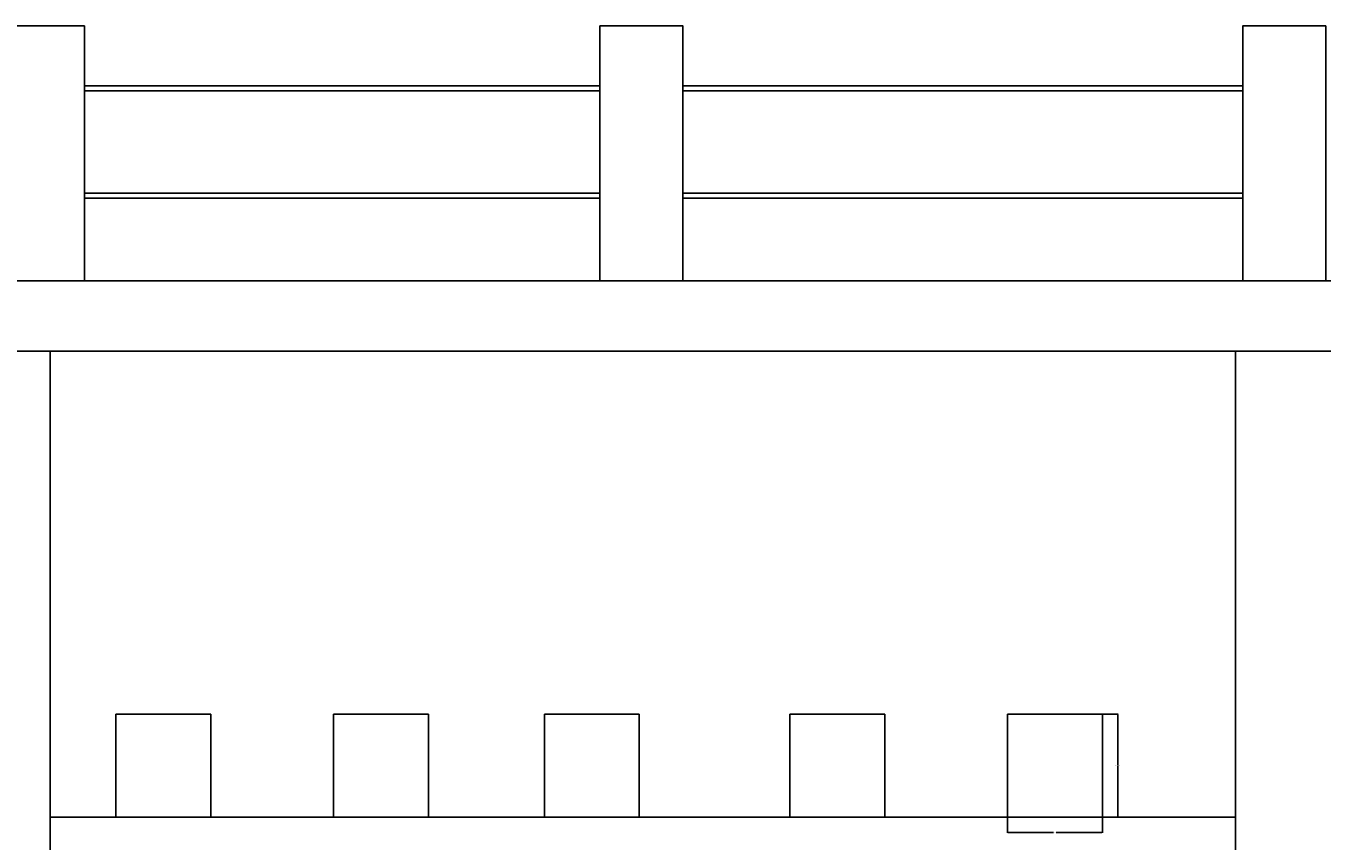
# Model space of a CAD drawing. Units: metres. Extents: x 10365 to 12529, y 3661 to 6248.
# Tile 8 of 9: x 11333 to 11858, y 5918 to 6248. Entities that reach past the tile are written whole.
import ezdxf

# ---------------------------------------------------------------- set-up
doc = ezdxf.new("R2010")
doc.units = ezdxf.units.M
doc.header["$MEASUREMENT"] = 0
doc.layers.add('A-ANNO-DIMS', color=2, linetype='Continuous', lineweight=18)
doc.layers.add('A-ELEV', color=7, linetype='Continuous', lineweight=25)
doc.styles.get("Standard").update_dxf_attribs({"font": 'arial.ttf'})
doc.dimstyles.get("Standard").update_dxf_attribs({"dimtxt": 0.18, "dimasz": 0.18, "dimexe": 0.18, "dimexo": 0.0625, "dimgap": 0.09, "dimtad": 0, "dimtih": 1, "dimtoh": 1, "dimdec": 0, "dimzin": 0, "dimdsep": 46, "dimtxsty": 'Standard', "dimcen": 0.09, "dimadec": 0, "dimazin": 0, "dimtfac": 1, "dimtdec": 0, "dimtofl": 0, "dimtmove": 0, "dimatfit": 3, "dimfxl": 1, "dimtolj": 1, "dimtzin": 0, "dimarcsym": 0})

# ---------------------------------------------------------------- blocks, each defined once
blk = doc.blocks.new('ELEV-PARAPET-BLOCK')
for p, q in [((0, 0), (0, 41.76)), ((0, 41.76), (38.46, 41.76)), ((38.46, 41.76), (38.46, 0))]:
    blk.add_line(p, q)
blk = doc.blocks.new('*D31')
at = {"layer": 'A-ANNO-DIMS', "color": 0, "lineweight": -2, "transparency": 16777216}
for p, q in [((11769.44, 5969.19), (11775.82, 5969.19)), ((11775.64, 5969.01), (11775.64, 5948.49)), ((11775.64, 5927.61), (11775.64, 5948.12)), ((11769.44, 5927.43), (11775.82, 5927.43))]:
    blk.add_line(p, q, dxfattribs=at)
at = {"layer": 'A-ANNO-DIMS', "color": 0, "transparency": 16777216}
for points in [[(11775.61, 5969.01), (11775.67, 5969.01), (11775.64, 5969.19)], [(11775.61, 5927.61), (11775.67, 5927.61), (11775.64, 5927.43)]]:
    blk.add_solid(points, dxfattribs=at)
at = {"layer": 'Defpoints', "color": 0, "transparency": 16777216}
for p in [(11769.38, 5969.19), (11775.64, 5969.19), (11769.38, 5927.43)]:
    blk.add_point(p, dxfattribs=at)
at = {"layer": 'A-ANNO-DIMS', "color": 0, "transparency": 16777216, "insert": (11775.64, 5948.31), "char_height": 0.18, "attachment_point": 5}
blk.add_mtext('\\A1;PARAPET BLOCK 42 TYP.', dxfattribs=at)
blk = doc.blocks.new('*D32')
at = {"layer": 'A-ANNO-DIMS', "color": 0, "lineweight": -2, "transparency": 16777216}
for p, q in [((11730.92, 5927.36), (11730.92, 5920.98)), ((11769.38, 5927.36), (11769.38, 5920.98)), ((11731.1, 5921.16), (11749.62, 5921.16)), ((11769.2, 5921.16), (11750.68, 5921.16))]:
    blk.add_line(p, q, dxfattribs=at)
at = {"layer": 'A-ANNO-DIMS', "color": 0, "transparency": 16777216}
for points in [[(11731.1, 5921.19), (11731.1, 5921.13), (11730.92, 5921.16)], [(11769.2, 5921.19), (11769.2, 5921.13), (11769.38, 5921.16)]]:
    blk.add_solid(points, dxfattribs=at)
at = {"layer": 'Defpoints', "color": 0, "transparency": 16777216}
for p in [(11730.92, 5927.43), (11769.38, 5927.43), (11769.38, 5921.16)]:
    blk.add_point(p, dxfattribs=at)
at = {"layer": 'A-ANNO-DIMS', "color": 0, "transparency": 16777216, "insert": (11750.15, 5921.16), "char_height": 0.18, "attachment_point": 5}
blk.add_mtext('\\A1;38 TYP.', dxfattribs=at)

msp = doc.modelspace()

# ---------------------------------------------------------------- linework, layer by layer
at = {"layer": 'A-ELEV'}
for p, q in [((11357.06, 6223.79), (11565.84, 6223.79)), ((11357.06, 6221.79), (11565.84, 6221.79)), ((11599.46, 6223.79), (11826.23, 6223.79)), ((11599.46, 6221.79), (11826.23, 6221.79)), ((11357.06, 6180.21), (11565.84, 6180.21)), ((11599.46, 6180.21), (11826.23, 6180.21)), ((11357.06, 6178.21), (11565.84, 6178.21)), ((11599.46, 6178.21), (11826.23, 6178.21)), ((11343.22, 5554.17), (11343.22, 6116.31)), ((11343.22, 6116.31), (12303.22, 6116.31)), ((11823.22, 6116.31), (11823.22, 5604.54)), ((11823.22, 5927.43), (11343.22, 5927.43))]:
    msp.add_line(p, q, dxfattribs=at)
for points in [[(11323.44, 6144.7), (11323.44, 6144.7), (11357.06, 6144.7), (11357.06, 6144.7), (11357.06, 6248.06), (11357.06, 6248.06), (11323.44, 6248.06), (11323.44, 6248.06)], [(11565.84, 6144.7), (11565.84, 6144.7), (11599.46, 6144.7), (11599.46, 6144.7), (11599.46, 6248.06), (11599.46, 6248.06), (11565.84, 6248.06), (11565.84, 6248.06)], [(11826.23, 6144.7), (11826.23, 6144.7), (11859.85, 6144.7), (11859.85, 6144.7), (11859.85, 6248.06), (11859.85, 6248.06), (11826.23, 6248.06), (11826.23, 6248.06)], [(11302.77, 6116.31), (11302.77, 6116.31), (12348.78, 6116.31), (12348.78, 6116.31), (12348.78, 6144.7), (12348.78, 6144.7), (11302.77, 6144.7), (11302.77, 6144.7)]]:
    msp.add_lwpolyline(points, close=True, dxfattribs=at)

# ---------------------------------------------------------------- block references
for p in [(11369.81, 5927.43), (11457.97, 5927.43), (11543.34, 5927.43), (11642.75, 5927.43), (11730.92, 5927.43)]:
    msp.add_blockref('ELEV-PARAPET-BLOCK', p, dxfattribs=at)

# ---------------------------------------------------------------- dimensions: what is measured, and where the dimension line sits
at = {"layer": 'A-ANNO-DIMS'}
dim = msp.add_linear_dim(base=(11775.64, 5969.19), p1=(11769.38, 5927.43), p2=(11769.38, 5969.19), angle=90, text='PARAPET BLOCK <> TYP.', dimstyle='Standard', override={"dimdec": 0, "dimrnd": 0, "dimzin": 0, "dimlunit": 2}, dxfattribs=at)
dim.commit()
dim.dimension.update_dxf_attribs({"geometry": '*D31', "text_midpoint": (11775.64, 5948.31)})
dim = msp.add_linear_dim(base=(11769.38, 5921.16), p1=(11730.92, 5927.43), p2=(11769.38, 5927.43), text='<> TYP.', dimstyle='Standard', override={"dimdec": 0, "dimrnd": 0, "dimzin": 0, "dimlunit": 2}, dxfattribs=at)
dim.commit()
dim.dimension.update_dxf_attribs({"geometry": '*D32', "text_midpoint": (11750.15, 5921.16)})

doc.saveas('drawing.dxf')
